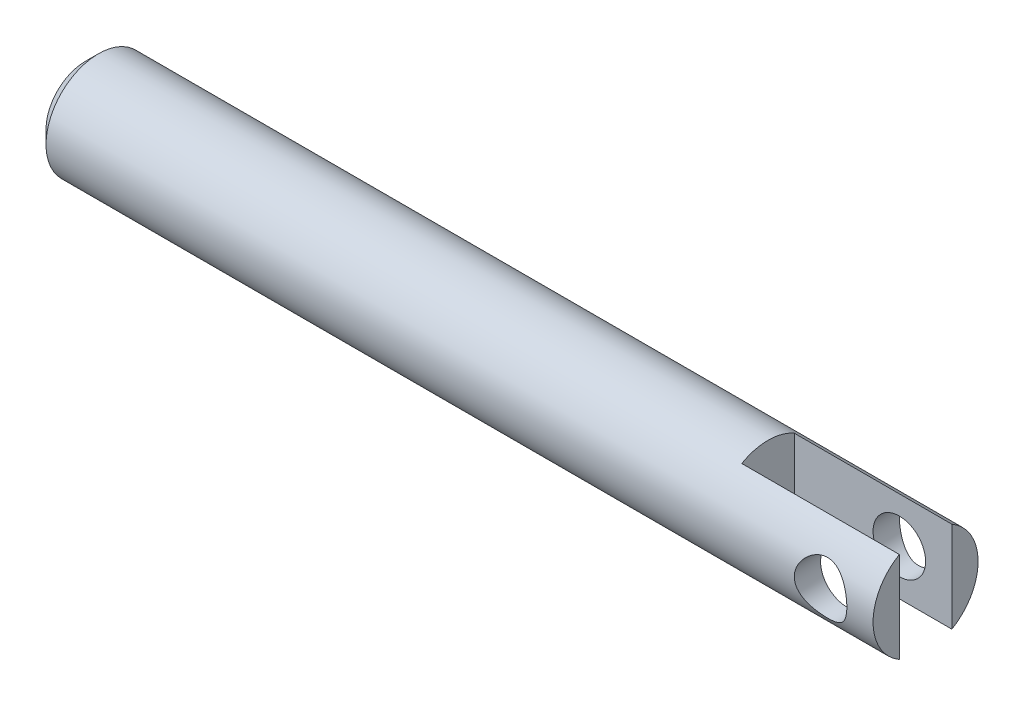
ISO-10303-21;
HEADER;
FILE_DESCRIPTION(('STEP AP214'),'2;1');
FILE_NAME('part.step','',(''),(''),'','','');
FILE_SCHEMA(('AUTOMOTIVE_DESIGN { 1 0 10303 214 1 1 1 1 }'));
ENDSEC;
DATA;
#1=APPLICATION_CONTEXT('core data for automotive mechanical design processes');
#2=APPLICATION_PROTOCOL_DEFINITION('international standard','automotive_design',2000,#1);
#3=PRODUCT_CONTEXT('',#1,'mechanical');
#4=PRODUCT('Part','Part','',(#3));
#5=PRODUCT_RELATED_PRODUCT_CATEGORY('part','',(#4));
#6=PRODUCT_DEFINITION_FORMATION('','',#4);
#7=PRODUCT_DEFINITION_CONTEXT('part definition',#1,'design');
#8=PRODUCT_DEFINITION('design','',#6,#7);
#9=PRODUCT_DEFINITION_SHAPE('','',#8);
#10=(LENGTH_UNIT() NAMED_UNIT(*) SI_UNIT(.MILLI.,.METRE.));
#11=(NAMED_UNIT(*) PLANE_ANGLE_UNIT() SI_UNIT($,.RADIAN.));
#12=(NAMED_UNIT(*) SI_UNIT($,.STERADIAN.) SOLID_ANGLE_UNIT());
#13=UNCERTAINTY_MEASURE_WITH_UNIT(LENGTH_MEASURE(1.E-05),#10,'distance_accuracy_value','');
#14=(GEOMETRIC_REPRESENTATION_CONTEXT(3) GLOBAL_UNCERTAINTY_ASSIGNED_CONTEXT((#13)) GLOBAL_UNIT_ASSIGNED_CONTEXT((#10,
#11,#12)) REPRESENTATION_CONTEXT('',''));
#15=CARTESIAN_POINT('',(0.,0.,0.));
#16=DIRECTION('',(0.,0.,1.));
#17=DIRECTION('',(1.,0.,0.));
#18=AXIS2_PLACEMENT_3D('',#15,#16,#17);
#19=CARTESIAN_POINT('',(50.8,6.35,0.));
#20=DIRECTION('',(-1.,0.,0.));
#21=DIRECTION('',(0.,0.,1.));
#22=AXIS2_PLACEMENT_3D('',#19,#20,#21);
#23=PLANE('',#22);
#24=CARTESIAN_POINT('',(50.8,0.,0.));
#25=DIRECTION('',(-1.,0.,0.));
#26=DIRECTION('',(0.,0.,1.));
#27=AXIS2_PLACEMENT_3D('',#24,#25,#26);
#28=CIRCLE('',#27,6.35);
#29=CARTESIAN_POINT('',(50.8,-5.49926131403119,3.175));
#30=VERTEX_POINT('',#29);
#31=CARTESIAN_POINT('',(50.8,5.49926131403119,3.175));
#32=VERTEX_POINT('',#31);
#33=EDGE_CURVE('E101',#30,#32,#28,.T.);
#34=ORIENTED_EDGE('',*,*,#33,.F.);
#35=DIRECTION('',(0.,1.,0.));
#36=VECTOR('',#35,1.);
#37=CARTESIAN_POINT('',(50.8,-127.,3.175));
#38=LINE('',#37,#36);
#39=EDGE_CURVE('E182',#30,#32,#38,.T.);
#40=ORIENTED_EDGE('',*,*,#39,.T.);
#41=EDGE_LOOP('',(#34,#40));
#42=FACE_BOUND('',#41,.T.);
#43=ADVANCED_FACE('F41',(#42),#23,.F.);
#44=CARTESIAN_POINT('',(44.45,0.,-127.));
#45=DIRECTION('',(0.,0.,1.));
#46=DIRECTION('',(1.,0.,0.));
#47=AXIS2_PLACEMENT_3D('',#44,#45,#46);
#48=CYLINDRICAL_SURFACE('',#47,3.175);
#49=CARTESIAN_POINT('',(44.45,0.,3.175));
#50=DIRECTION('',(0.,0.,1.));
#51=DIRECTION('',(1.,0.,0.));
#52=AXIS2_PLACEMENT_3D('',#49,#50,#51);
#53=CIRCLE('',#52,3.175);
#54=CARTESIAN_POINT('',(47.625,0.,3.175));
#55=VERTEX_POINT('',#54);
#56=EDGE_CURVE('E90',#55,#55,#53,.F.);
#57=ORIENTED_EDGE('',*,*,#56,.T.);
#58=EDGE_LOOP('',(#57));
#59=FACE_BOUND('',#58,.T.);
#60=CARTESIAN_POINT('',(47.625,0.,6.35));
#61=CARTESIAN_POINT('',(47.6249991122824,-0.0834969220595001,6.34999931166444));
#62=CARTESIAN_POINT('',(47.6217001255541,-0.167002655580043,6.34834758911701));
#63=CARTESIAN_POINT('',(47.6085541254501,-0.333378330258782,6.34179105821714));
#64=CARTESIAN_POINT('',(47.5987042634742,-0.416247978955772,6.33688483467113));
#65=CARTESIAN_POINT('',(47.559427934954,-0.66318203064701,6.31742426748325));
#66=CARTESIAN_POINT('',(47.5202749225986,-0.825450146761553,6.29812827299425));
#67=CARTESIAN_POINT('',(47.4180092887059,-1.13965128900426,6.2489182313574));
#68=CARTESIAN_POINT('',(47.3549897807566,-1.29162180811868,6.21904547786825));
#69=CARTESIAN_POINT('',(47.2072639263711,-1.58264035037879,6.15142812041637));
#70=CARTESIAN_POINT('',(47.1225592898491,-1.72168939123018,6.11368413715877));
#71=CARTESIAN_POINT('',(46.9280303702658,-1.99234108848171,6.03111096182982));
#72=CARTESIAN_POINT('',(46.8169964222061,-2.12298433900091,5.98599127270818));
#73=CARTESIAN_POINT('',(46.5756033164272,-2.36467069069853,5.89470535591056));
#74=CARTESIAN_POINT('',(46.4452295702336,-2.47569885601321,5.84853836069043));
#75=CARTESIAN_POINT('',(46.1565790522467,-2.68368848497886,5.75623634934464));
#76=CARTESIAN_POINT('',(45.9969224686984,-2.77889135161933,5.71038146176788));
#77=CARTESIAN_POINT('',(45.7454520128256,-2.90019349951534,5.64919759286363));
#78=CARTESIAN_POINT('',(45.6595999381713,-2.93705266116891,5.63006420805933));
#79=CARTESIAN_POINT('',(45.4844143862936,-3.00322508739606,5.59504604853268));
#80=CARTESIAN_POINT('',(45.3950830018195,-3.03254280972159,5.57915935583429));
#81=CARTESIAN_POINT('',(45.2189894480353,-3.08174263292982,5.55212611635049));
#82=CARTESIAN_POINT('',(45.1323892059714,-3.10208128111978,5.54075429137746));
#83=CARTESIAN_POINT('',(44.9574127210056,-3.13545600360765,5.52193654886444));
#84=CARTESIAN_POINT('',(44.8690374462283,-3.14849595237257,5.51448854851135));
#85=CARTESIAN_POINT('',(44.6912932611514,-3.1670771305344,5.50383875782919));
#86=CARTESIAN_POINT('',(44.6019249820126,-3.17262287599649,5.50063441026522));
#87=CARTESIAN_POINT('',(44.4230192158219,-3.17614778806993,5.49859788398609));
#88=CARTESIAN_POINT('',(44.3334817457287,-3.17412767659872,5.49976528812799));
#89=CARTESIAN_POINT('',(44.0872521242756,-3.1581193033026,5.50899190362733));
#90=CARTESIAN_POINT('',(43.9311582701866,-3.13621253452965,5.52160857357707));
#91=CARTESIAN_POINT('',(43.6253533586935,-3.07003746372167,5.55866493052824));
#92=CARTESIAN_POINT('',(43.4756443509772,-3.02576203854504,5.58310838358077));
#93=CARTESIAN_POINT('',(43.1824557034359,-2.91531509833647,5.64157885407237));
#94=CARTESIAN_POINT('',(43.0392023900634,-2.84865758129417,5.67581583876129));
#95=CARTESIAN_POINT('',(42.765233913826,-2.69570761526054,5.75003268807633));
#96=CARTESIAN_POINT('',(42.6345244203915,-2.60940634674629,5.79001512927804));
#97=CARTESIAN_POINT('',(42.3718957257497,-2.40685964249565,5.87734289018611));
#98=CARTESIAN_POINT('',(42.2419246151435,-2.28820488335253,5.92497898403936));
#99=CARTESIAN_POINT('',(42.0029148571362,-2.03058898448427,6.01813700574905));
#100=CARTESIAN_POINT('',(41.8938862136413,-1.89161819563546,6.06365791538158));
#101=CARTESIAN_POINT('',(41.6950980802803,-1.58913989972482,6.1500381059768));
#102=CARTESIAN_POINT('',(41.6064685144201,-1.42479265164789,6.19058274974572));
#103=CARTESIAN_POINT('',(41.4588419183647,-1.08098023585583,6.25976272299952));
#104=CARTESIAN_POINT('',(41.3998213588683,-0.901527205073898,6.28840750578946));
#105=CARTESIAN_POINT('',(41.317940596601,-0.548533610626836,6.32854759690358));
#106=CARTESIAN_POINT('',(41.2924903274127,-0.375734359385247,6.34126679122995));
#107=CARTESIAN_POINT('',(41.2703494777398,-0.0278752299448333,6.35231817716325));
#108=CARTESIAN_POINT('',(41.2736452728607,0.147183538060018,6.35065718436129));
#109=CARTESIAN_POINT('',(41.3074062359454,0.480164686080362,6.33384535408399));
#110=CARTESIAN_POINT('',(41.3357457914748,0.638363620564189,6.31975005060431));
#111=CARTESIAN_POINT('',(41.4154558782099,0.947441883053,6.28085393924121));
#112=CARTESIAN_POINT('',(41.4668289484773,1.09832040207141,6.25605195113515));
#113=CARTESIAN_POINT('',(41.5924951309378,1.39347133182512,6.19709998236334));
#114=CARTESIAN_POINT('',(41.6674015841112,1.53743151047821,6.16270299610718));
#115=CARTESIAN_POINT('',(41.8373164256859,1.8112148234104,6.08787118465665));
#116=CARTESIAN_POINT('',(41.9323333773854,1.94103189959927,6.0474337895468));
#117=CARTESIAN_POINT('',(42.1505393503738,2.19636241342679,5.95973602709939));
#118=CARTESIAN_POINT('',(42.2755786071116,2.3202013468198,5.91219559251098));
#119=CARTESIAN_POINT('',(42.5447623551498,2.54589381918873,5.81858093231368));
#120=CARTESIAN_POINT('',(42.6889199523809,2.6477321493525,5.77250773963547));
#121=CARTESIAN_POINT('',(43.0010686019584,2.83117262876715,5.68487535288742));
#122=CARTESIAN_POINT('',(43.1698757695104,2.91155594998013,5.64364281441821));
#123=CARTESIAN_POINT('',(43.5213444648897,3.04191297152938,5.5744767953732));
#124=CARTESIAN_POINT('',(43.7039877978474,3.09192585492219,5.54652618900869));
#125=CARTESIAN_POINT('',(44.0591899564702,3.15551086037918,5.51057765714603));
#126=CARTESIAN_POINT('',(44.2310337504072,3.17212027309711,5.50092192343245));
#127=CARTESIAN_POINT('',(44.5752444424952,3.17718805563876,5.49800001145358));
#128=CARTESIAN_POINT('',(44.7476110815426,3.16565862768385,5.5047267290444));
#129=CARTESIAN_POINT('',(45.0706601030739,3.11761548073658,5.53205211477784));
#130=CARTESIAN_POINT('',(45.2218439417312,3.08358651207686,5.55126823076269));
#131=CARTESIAN_POINT('',(45.5161908301672,2.99458164828807,5.59977978302582));
#132=CARTESIAN_POINT('',(45.6593512828503,2.93959901505999,5.62907846127335));
#133=CARTESIAN_POINT('',(45.9442336994286,2.8061154442137,5.69685576337174));
#134=CARTESIAN_POINT('',(46.0852128093657,2.72628260503929,5.73581889480533));
#135=CARTESIAN_POINT('',(46.3526974317231,2.54682759156583,5.81772207082382));
#136=CARTESIAN_POINT('',(46.4791953599427,2.44719512169931,5.8606641782013));
#137=CARTESIAN_POINT('',(46.7300975241771,2.21680287661218,5.95192753761204));
#138=CARTESIAN_POINT('',(46.8523797564128,2.08373188558712,6.00026839877346));
#139=CARTESIAN_POINT('',(47.0733978732331,1.79751265125243,6.0921234557675));
#140=CARTESIAN_POINT('',(47.1721210659827,1.64435365457428,6.13563504323043));
#141=CARTESIAN_POINT('',(47.3002802661971,1.40178715704487,6.19391073190243));
#142=CARTESIAN_POINT('',(47.3398005836814,1.31842200030918,6.21223173271383));
#143=CARTESIAN_POINT('',(47.4115994748237,1.1480770102167,6.24595363475604));
#144=CARTESIAN_POINT('',(47.4438816065344,1.06109897786306,6.26135597012704));
#145=CARTESIAN_POINT('',(47.500759345915,0.884361322813108,6.28875097111981));
#146=CARTESIAN_POINT('',(47.5253717181381,0.794608244970572,6.30075106809478));
#147=CARTESIAN_POINT('',(47.5666673895299,0.612925661591583,6.32100983571903));
#148=CARTESIAN_POINT('',(47.5833555321936,0.520997521680291,6.3292707916836));
#149=CARTESIAN_POINT('',(47.6056162848624,0.357531347524375,6.34032503263334));
#150=CARTESIAN_POINT('',(47.6128788212496,0.286274046488596,6.34394670812889));
#151=CARTESIAN_POINT('',(47.6225711265376,0.143346668941346,6.34878452045567));
#152=CARTESIAN_POINT('',(47.6250007620468,0.0716765810914255,6.35000059089052));
#153=CARTESIAN_POINT('',(47.625,0.,6.35));
#154=B_SPLINE_CURVE_WITH_KNOTS('',3,(#60,#61,#62,#63,#64,#65,#66,#67,#68,#69,#70,#71,#72,#73,
#74,#75,#76,#77,#78,#79,#80,#81,#82,#83,#84,#85,#86,#87,#88,#89,#90,#91,#92,#93,#94,#95,#96,#97,
#98,#99,#100,#101,#102,#103,#104,#105,#106,#107,#108,#109,#110,#111,#112,#113,#114,#115,#116,
#117,#118,#119,#120,#121,#122,#123,#124,#125,#126,#127,#128,#129,#130,#131,#132,#133,#134,#135,
#136,#137,#138,#139,#140,#141,#142,#143,#144,#145,#146,#147,#148,#149,#150,#151,#152,#153),
.UNSPECIFIED.,.T.,.F.,(4,2,2,2,2,2,2,2,2,2,2,2,2,2,2,2,2,2,2,2,2,2,2,2,2,2,2,2,2,2,2,2,2,2,2,2,
2,2,2,2,2,2,2,2,2,2,4),(0.,0.25041561210268,0.500940186864015,1.00234854488129,1.50182051324263,
2.00125310940106,2.53090025348451,3.06094897410615,3.63210298373097,3.91787290005988,
4.20347350732849,4.47213270490101,4.74064915090146,5.00900371453886,5.27733267302576,
5.74927594687738,6.22136960256845,6.70445970327764,7.18776712794021,7.7323564652788,
8.27720530143645,8.84735553323665,9.41705196489304,9.93956405039338,10.4618285011675,
10.9436138594975,11.4254523397102,11.9210677568139,12.4168946391879,12.9614122158798,
13.5063050164601,14.0775857365549,14.6481278321882,15.1639000911419,15.6794487286237,
16.1458838633213,16.6124691169503,17.1104020806943,17.6085946442304,18.1673210354482,
18.7263477502426,19.0082017078365,19.2899168101042,19.5710117490933,19.8519346536844,
20.0668939492148,20.2818591776892),.UNSPECIFIED.);
#155=CARTESIAN_POINT('',(47.625,0.,6.35));
#156=VERTEX_POINT('',#155);
#157=EDGE_CURVE('E106',#156,#156,#154,.T.);
#158=ORIENTED_EDGE('',*,*,#157,.F.);
#159=EDGE_LOOP('',(#158));
#160=FACE_BOUND('',#159,.T.);
#161=ADVANCED_FACE('F128',(#59,#160),#48,.F.);
#162=CARTESIAN_POINT('',(-50.8,6.35,0.));
#163=DIRECTION('',(1.,0.,0.));
#164=DIRECTION('',(0.,0.,-1.));
#165=AXIS2_PLACEMENT_3D('',#162,#163,#164);
#166=PLANE('',#165);
#167=CARTESIAN_POINT('',(-50.8,0.,0.));
#168=DIRECTION('',(1.,0.,0.));
#169=DIRECTION('',(0.,0.,-1.));
#170=AXIS2_PLACEMENT_3D('',#167,#168,#169);
#171=CIRCLE('',#170,4.76249999999999);
#172=CARTESIAN_POINT('',(-50.8,0.,-4.76249999999999));
#173=VERTEX_POINT('',#172);
#174=EDGE_CURVE('E47',#173,#173,#171,.F.);
#175=ORIENTED_EDGE('',*,*,#174,.T.);
#176=EDGE_LOOP('',(#175));
#177=FACE_BOUND('',#176,.T.);
#178=CARTESIAN_POINT('',(-50.8,0.,0.));
#179=DIRECTION('',(-1.,0.,0.));
#180=DIRECTION('',(0.,0.,1.));
#181=AXIS2_PLACEMENT_3D('',#178,#179,#180);
#182=CIRCLE('',#181,3.96875);
#183=CARTESIAN_POINT('',(-50.8,0.,3.96875));
#184=VERTEX_POINT('',#183);
#185=EDGE_CURVE('E176',#184,#184,#182,.T.);
#186=ORIENTED_EDGE('',*,*,#185,.F.);
#187=EDGE_LOOP('',(#186));
#188=FACE_BOUND('',#187,.T.);
#189=ADVANCED_FACE('F157',(#177,#188),#166,.F.);
#190=CARTESIAN_POINT('',(50.8,5.49926131403119,-3.175));
#191=VERTEX_POINT('',#190);
#192=CARTESIAN_POINT('',(50.8,-5.49926131403119,-3.175));
#193=VERTEX_POINT('',#192);
#194=EDGE_CURVE('E92',#191,#193,#28,.T.);
#195=ORIENTED_EDGE('',*,*,#194,.F.);
#196=DIRECTION('',(0.,1.,0.));
#197=VECTOR('',#196,1.);
#198=CARTESIAN_POINT('',(50.8,-127.,-3.175));
#199=LINE('',#198,#197);
#200=EDGE_CURVE('E57',#193,#191,#199,.T.);
#201=ORIENTED_EDGE('',*,*,#200,.F.);
#202=EDGE_LOOP('',(#195,#201));
#203=FACE_BOUND('',#202,.T.);
#204=ADVANCED_FACE('F94',(#203),#23,.F.);
#205=CARTESIAN_POINT('',(-58.2524572001112,0.,0.));
#206=DIRECTION('',(-1.,0.,0.));
#207=DIRECTION('',(0.,0.,1.));
#208=AXIS2_PLACEMENT_3D('',#205,#206,#207);
#209=CYLINDRICAL_SURFACE('',#208,6.35);
#210=CARTESIAN_POINT('',(-49.2125,0.,0.));
#211=DIRECTION('',(1.,0.,0.));
#212=DIRECTION('',(0.,0.,-1.));
#213=AXIS2_PLACEMENT_3D('',#210,#211,#212);
#214=CIRCLE('',#213,6.35);
#215=CARTESIAN_POINT('',(-49.2125,0.,-6.35));
#216=VERTEX_POINT('',#215);
#217=EDGE_CURVE('E11',#216,#216,#214,.T.);
#218=ORIENTED_EDGE('',*,*,#217,.T.);
#219=EDGE_LOOP('',(#218));
#220=FACE_BOUND('',#219,.T.);
#221=ORIENTED_EDGE('',*,*,#157,.T.);
#222=EDGE_LOOP('',(#221));
#223=FACE_BOUND('',#222,.T.);
#224=CARTESIAN_POINT('',(47.625,0.,-6.35));
#225=CARTESIAN_POINT('',(47.6249991122824,0.0834969220594997,-6.34999931166444));
#226=CARTESIAN_POINT('',(47.6217001255541,0.167002655580042,-6.34834758911701));
#227=CARTESIAN_POINT('',(47.6085541254501,0.333378330258781,-6.34179105821715));
#228=CARTESIAN_POINT('',(47.5987042634742,0.416247978955771,-6.33688483467113));
#229=CARTESIAN_POINT('',(47.559427934954,0.663182030647009,-6.31742426748325));
#230=CARTESIAN_POINT('',(47.5202749225986,0.825450146761553,-6.29812827299425));
#231=CARTESIAN_POINT('',(47.4180092887059,1.13965128900426,-6.2489182313574));
#232=CARTESIAN_POINT('',(47.3549897807566,1.29162180811868,-6.21904547786825));
#233=CARTESIAN_POINT('',(47.2072639263711,1.58264035037879,-6.15142812041637));
#234=CARTESIAN_POINT('',(47.1225592898491,1.72168939123018,-6.11368413715877));
#235=CARTESIAN_POINT('',(46.9280303702658,1.99234108848171,-6.03111096182982));
#236=CARTESIAN_POINT('',(46.8169964222061,2.12298433900091,-5.98599127270818));
#237=CARTESIAN_POINT('',(46.5756033164272,2.36467069069853,-5.89470535591056));
#238=CARTESIAN_POINT('',(46.4452295702336,2.47569885601321,-5.84853836069043));
#239=CARTESIAN_POINT('',(46.1565790522467,2.68368848497886,-5.75623634934464));
#240=CARTESIAN_POINT('',(45.9969224686984,2.77889135161933,-5.71038146176788));
#241=CARTESIAN_POINT('',(45.7454520128256,2.90019349951534,-5.64919759286363));
#242=CARTESIAN_POINT('',(45.6595999381713,2.93705266116891,-5.63006420805933));
#243=CARTESIAN_POINT('',(45.4844143862936,3.00322508739606,-5.59504604853268));
#244=CARTESIAN_POINT('',(45.3950830018195,3.03254280972159,-5.57915935583429));
#245=CARTESIAN_POINT('',(45.2189894480353,3.08174263292982,-5.55212611635049));
#246=CARTESIAN_POINT('',(45.1323892059714,3.10208128111978,-5.54075429137746));
#247=CARTESIAN_POINT('',(44.9574127210056,3.13545600360765,-5.52193654886444));
#248=CARTESIAN_POINT('',(44.8690374462283,3.14849595237257,-5.51448854851135));
#249=CARTESIAN_POINT('',(44.6912932611514,3.1670771305344,-5.50383875782919));
#250=CARTESIAN_POINT('',(44.6019249820126,3.17262287599649,-5.50063441026522));
#251=CARTESIAN_POINT('',(44.4230192158219,3.17614778806993,-5.49859788398609));
#252=CARTESIAN_POINT('',(44.3334817457287,3.17412767659872,-5.49976528812799));
#253=CARTESIAN_POINT('',(44.0872521242756,3.1581193033026,-5.50899190362733));
#254=CARTESIAN_POINT('',(43.9311582701866,3.13621253452965,-5.52160857357707));
#255=CARTESIAN_POINT('',(43.6253533586935,3.07003746372167,-5.55866493052824));
#256=CARTESIAN_POINT('',(43.4756443509772,3.02576203854504,-5.58310838358077));
#257=CARTESIAN_POINT('',(43.1824557034359,2.91531509833647,-5.64157885407237));
#258=CARTESIAN_POINT('',(43.0392023900634,2.84865758129417,-5.67581583876129));
#259=CARTESIAN_POINT('',(42.765233913826,2.69570761526054,-5.75003268807633));
#260=CARTESIAN_POINT('',(42.6345244203915,2.60940634674629,-5.79001512927804));
#261=CARTESIAN_POINT('',(42.3718957257497,2.40685964249565,-5.87734289018611));
#262=CARTESIAN_POINT('',(42.2419246151435,2.28820488335253,-5.92497898403936));
#263=CARTESIAN_POINT('',(42.0029148571362,2.03058898448427,-6.01813700574905));
#264=CARTESIAN_POINT('',(41.8938862136413,1.89161819563546,-6.06365791538158));
#265=CARTESIAN_POINT('',(41.6950980802803,1.58913989972482,-6.1500381059768));
#266=CARTESIAN_POINT('',(41.6064685144201,1.42479265164789,-6.19058274974572));
#267=CARTESIAN_POINT('',(41.4588419183647,1.08098023585583,-6.25976272299952));
#268=CARTESIAN_POINT('',(41.3998213588683,0.901527205073898,-6.28840750578946));
#269=CARTESIAN_POINT('',(41.317940596601,0.548533610626835,-6.32854759690358));
#270=CARTESIAN_POINT('',(41.2924903274127,0.375734359385245,-6.34126679122995));
#271=CARTESIAN_POINT('',(41.2703494777398,0.0278752299448316,-6.35231817716325));
#272=CARTESIAN_POINT('',(41.2736452728607,-0.147183538060019,-6.35065718436129));
#273=CARTESIAN_POINT('',(41.3074062359454,-0.480164686080362,-6.33384535408399));
#274=CARTESIAN_POINT('',(41.3357457914748,-0.63836362056419,-6.31975005060431));
#275=CARTESIAN_POINT('',(41.4154558782099,-0.947441883053001,-6.28085393924121));
#276=CARTESIAN_POINT('',(41.4668289484773,-1.09832040207141,-6.25605195113515));
#277=CARTESIAN_POINT('',(41.5924951309378,-1.39347133182512,-6.19709998236334));
#278=CARTESIAN_POINT('',(41.6674015841112,-1.53743151047822,-6.16270299610718));
#279=CARTESIAN_POINT('',(41.8373164256859,-1.8112148234104,-6.08787118465664));
#280=CARTESIAN_POINT('',(41.9323333773854,-1.94103189959927,-6.0474337895468));
#281=CARTESIAN_POINT('',(42.1505393503738,-2.19636241342679,-5.95973602709939));
#282=CARTESIAN_POINT('',(42.2755786071116,-2.3202013468198,-5.91219559251098));
#283=CARTESIAN_POINT('',(42.5447623551498,-2.54589381918874,-5.81858093231368));
#284=CARTESIAN_POINT('',(42.6889199523809,-2.64773214935251,-5.77250773963547));
#285=CARTESIAN_POINT('',(43.0010686019584,-2.83117262876716,-5.68487535288742));
#286=CARTESIAN_POINT('',(43.1698757695104,-2.91155594998014,-5.64364281441821));
#287=CARTESIAN_POINT('',(43.5213444648897,-3.04191297152938,-5.5744767953732));
#288=CARTESIAN_POINT('',(43.7039877978474,-3.09192585492219,-5.54652618900869));
#289=CARTESIAN_POINT('',(44.0591899564702,-3.15551086037918,-5.51057765714603));
#290=CARTESIAN_POINT('',(44.2310337504072,-3.17212027309711,-5.50092192343245));
#291=CARTESIAN_POINT('',(44.5752444424952,-3.17718805563876,-5.49800001145358));
#292=CARTESIAN_POINT('',(44.7476110815427,-3.16565862768385,-5.50472672904441));
#293=CARTESIAN_POINT('',(45.0706601030739,-3.11761548073657,-5.53205211477784));
#294=CARTESIAN_POINT('',(45.2218439417312,-3.08358651207686,-5.55126823076269));
#295=CARTESIAN_POINT('',(45.5161908301672,-2.99458164828807,-5.59977978302582));
#296=CARTESIAN_POINT('',(45.6593512828503,-2.93959901505999,-5.62907846127335));
#297=CARTESIAN_POINT('',(45.9442336994286,-2.8061154442137,-5.69685576337174));
#298=CARTESIAN_POINT('',(46.0852128093657,-2.72628260503929,-5.73581889480533));
#299=CARTESIAN_POINT('',(46.3526974317231,-2.54682759156583,-5.81772207082382));
#300=CARTESIAN_POINT('',(46.4791953599427,-2.44719512169931,-5.8606641782013));
#301=CARTESIAN_POINT('',(46.7300975241771,-2.21680287661218,-5.95192753761204));
#302=CARTESIAN_POINT('',(46.8523797564128,-2.08373188558712,-6.00026839877347));
#303=CARTESIAN_POINT('',(47.0733978732331,-1.79751265125243,-6.0921234557675));
#304=CARTESIAN_POINT('',(47.1721210659827,-1.64435365457428,-6.13563504323043));
#305=CARTESIAN_POINT('',(47.3002802661971,-1.40178715704487,-6.19391073190243));
#306=CARTESIAN_POINT('',(47.3398005836814,-1.31842200030918,-6.21223173271383));
#307=CARTESIAN_POINT('',(47.4115994748237,-1.1480770102167,-6.24595363475604));
#308=CARTESIAN_POINT('',(47.4438816065344,-1.06109897786306,-6.26135597012704));
#309=CARTESIAN_POINT('',(47.500759345915,-0.884361322813107,-6.28875097111981));
#310=CARTESIAN_POINT('',(47.5253717181381,-0.79460824497057,-6.30075106809478));
#311=CARTESIAN_POINT('',(47.5666673895299,-0.61292566159158,-6.32100983571903));
#312=CARTESIAN_POINT('',(47.5833555321936,-0.520997521680289,-6.3292707916836));
#313=CARTESIAN_POINT('',(47.6056162848624,-0.357531347524375,-6.34032503263334));
#314=CARTESIAN_POINT('',(47.6128788212496,-0.286274046488597,-6.34394670812889));
#315=CARTESIAN_POINT('',(47.6225711265376,-0.143346668941348,-6.34878452045567));
#316=CARTESIAN_POINT('',(47.6250007620468,-0.0716765810914264,-6.35000059089052));
#317=CARTESIAN_POINT('',(47.625,0.,-6.35));
#318=B_SPLINE_CURVE_WITH_KNOTS('',3,(#224,#225,#226,#227,#228,#229,#230,#231,#232,#233,#234,
#235,#236,#237,#238,#239,#240,#241,#242,#243,#244,#245,#246,#247,#248,#249,#250,#251,#252,#253,
#254,#255,#256,#257,#258,#259,#260,#261,#262,#263,#264,#265,#266,#267,#268,#269,#270,#271,#272,
#273,#274,#275,#276,#277,#278,#279,#280,#281,#282,#283,#284,#285,#286,#287,#288,#289,#290,#291,
#292,#293,#294,#295,#296,#297,#298,#299,#300,#301,#302,#303,#304,#305,#306,#307,#308,#309,#310,
#311,#312,#313,#314,#315,#316,#317),.UNSPECIFIED.,.T.,.F.,(4,2,2,2,2,2,2,2,2,2,2,2,2,2,2,2,2,2,
2,2,2,2,2,2,2,2,2,2,2,2,2,2,2,2,2,2,2,2,2,2,2,2,2,2,2,2,4),(0.,0.25041561210268,
0.500940186864013,1.00234854488129,1.50182051324263,2.00125310940106,2.53090025348452,
3.06094897410615,3.63210298373097,3.91787290005988,4.20347350732849,4.47213270490101,
4.74064915090146,5.00900371453886,5.27733267302576,5.74927594687738,6.22136960256845,
6.70445970327764,7.18776712794021,7.7323564652788,8.27720530143645,8.84735553323665,
9.41705196489304,9.93956405039339,10.4618285011675,10.9436138594975,11.4254523397102,
11.9210677568139,12.4168946391879,12.9614122158798,13.5063050164601,14.0775857365549,
14.6481278321882,15.1639000911419,15.6794487286237,16.1458838633213,16.6124691169503,
17.1104020806943,17.6085946442304,18.1673210354482,18.7263477502426,19.0082017078365,
19.2899168101042,19.5710117490933,19.8519346536844,20.0668939492147,20.2818591776892),.UNSPECIFIED.);
#319=CARTESIAN_POINT('',(47.625,0.,-6.35));
#320=VERTEX_POINT('',#319);
#321=EDGE_CURVE('E109',#320,#320,#318,.T.);
#322=ORIENTED_EDGE('',*,*,#321,.T.);
#323=EDGE_LOOP('',(#322));
#324=FACE_BOUND('',#323,.T.);
#325=CARTESIAN_POINT('',(31.75,0.,0.));
#326=DIRECTION('',(-1.,0.,0.));
#327=DIRECTION('',(0.,0.,1.));
#328=AXIS2_PLACEMENT_3D('',#325,#326,#327);
#329=CIRCLE('',#328,6.35);
#330=CARTESIAN_POINT('',(31.75,-5.49926131403119,-3.175));
#331=VERTEX_POINT('',#330);
#332=CARTESIAN_POINT('',(31.75,-5.49926131403118,3.175));
#333=VERTEX_POINT('',#332);
#334=EDGE_CURVE('E103',#331,#333,#329,.T.);
#335=ORIENTED_EDGE('',*,*,#334,.T.);
#336=DIRECTION('',(-1.,0.,0.));
#337=VECTOR('',#336,1.);
#338=CARTESIAN_POINT('',(-58.2524572001112,-5.49926131403118,3.175));
#339=LINE('',#338,#337);
#340=EDGE_CURVE('E190',#333,#30,#339,.F.);
#341=ORIENTED_EDGE('',*,*,#340,.T.);
#342=ORIENTED_EDGE('',*,*,#33,.T.);
#343=DIRECTION('',(-1.,0.,0.));
#344=VECTOR('',#343,1.);
#345=CARTESIAN_POINT('',(-58.2524572001112,5.49926131403118,3.175));
#346=LINE('',#345,#344);
#347=CARTESIAN_POINT('',(31.75,5.49926131403118,3.175));
#348=VERTEX_POINT('',#347);
#349=EDGE_CURVE('E64',#32,#348,#346,.T.);
#350=ORIENTED_EDGE('',*,*,#349,.T.);
#351=CARTESIAN_POINT('',(31.75,5.49926131403119,-3.175));
#352=VERTEX_POINT('',#351);
#353=EDGE_CURVE('E99',#348,#352,#329,.T.);
#354=ORIENTED_EDGE('',*,*,#353,.T.);
#355=DIRECTION('',(-1.,0.,0.));
#356=VECTOR('',#355,1.);
#357=CARTESIAN_POINT('',(-58.2524572001112,5.49926131403119,-3.175));
#358=LINE('',#357,#356);
#359=EDGE_CURVE('E89',#352,#191,#358,.F.);
#360=ORIENTED_EDGE('',*,*,#359,.T.);
#361=ORIENTED_EDGE('',*,*,#194,.T.);
#362=DIRECTION('',(-1.,0.,0.));
#363=VECTOR('',#362,1.);
#364=CARTESIAN_POINT('',(-58.2524572001112,-5.49926131403119,-3.175));
#365=LINE('',#364,#363);
#366=EDGE_CURVE('E85',#193,#331,#365,.T.);
#367=ORIENTED_EDGE('',*,*,#366,.T.);
#368=EDGE_LOOP('',(#335,#341,#342,#350,#354,#360,#361,#367));
#369=FACE_BOUND('',#368,.T.);
#370=ADVANCED_FACE('F98',(#220,#223,#324,#369),#209,.T.);
#371=CARTESIAN_POINT('',(44.45,0.,-3.175));
#372=DIRECTION('',(0.,0.,-1.));
#373=DIRECTION('',(-1.,0.,0.));
#374=AXIS2_PLACEMENT_3D('',#371,#372,#373);
#375=CIRCLE('',#374,3.175);
#376=CARTESIAN_POINT('',(41.275,0.,-3.175));
#377=VERTEX_POINT('',#376);
#378=EDGE_CURVE('E181',#377,#377,#375,.F.);
#379=ORIENTED_EDGE('',*,*,#378,.T.);
#380=EDGE_LOOP('',(#379));
#381=FACE_BOUND('',#380,.T.);
#382=ORIENTED_EDGE('',*,*,#321,.F.);
#383=EDGE_LOOP('',(#382));
#384=FACE_BOUND('',#383,.T.);
#385=ADVANCED_FACE('F123',(#381,#384),#48,.F.);
#386=CARTESIAN_POINT('',(31.75,-127.,3.175));
#387=DIRECTION('',(-1.,0.,0.));
#388=DIRECTION('',(0.,0.,1.));
#389=AXIS2_PLACEMENT_3D('',#386,#387,#388);
#390=PLANE('',#389);
#391=DIRECTION('',(0.,1.,0.));
#392=VECTOR('',#391,1.);
#393=CARTESIAN_POINT('',(31.75,-127.,3.175));
#394=LINE('',#393,#392);
#395=EDGE_CURVE('E184',#333,#348,#394,.T.);
#396=ORIENTED_EDGE('',*,*,#395,.F.);
#397=ORIENTED_EDGE('',*,*,#334,.F.);
#398=DIRECTION('',(0.,1.,0.));
#399=VECTOR('',#398,1.);
#400=CARTESIAN_POINT('',(31.75,-127.,-3.175));
#401=LINE('',#400,#399);
#402=EDGE_CURVE('E84',#331,#352,#401,.T.);
#403=ORIENTED_EDGE('',*,*,#402,.T.);
#404=ORIENTED_EDGE('',*,*,#353,.F.);
#405=EDGE_LOOP('',(#396,#397,#403,#404));
#406=FACE_BOUND('',#405,.T.);
#407=ADVANCED_FACE('F126',(#406),#390,.F.);
#408=CARTESIAN_POINT('',(31.75,-127.,3.175));
#409=DIRECTION('',(0.,0.,1.));
#410=DIRECTION('',(1.,0.,0.));
#411=AXIS2_PLACEMENT_3D('',#408,#409,#410);
#412=PLANE('',#411);
#413=ORIENTED_EDGE('',*,*,#56,.F.);
#414=EDGE_LOOP('',(#413));
#415=FACE_BOUND('',#414,.T.);
#416=ORIENTED_EDGE('',*,*,#39,.F.);
#417=ORIENTED_EDGE('',*,*,#340,.F.);
#418=ORIENTED_EDGE('',*,*,#395,.T.);
#419=ORIENTED_EDGE('',*,*,#349,.F.);
#420=EDGE_LOOP('',(#416,#417,#418,#419));
#421=FACE_BOUND('',#420,.T.);
#422=ADVANCED_FACE('F132',(#415,#421),#412,.F.);
#423=CARTESIAN_POINT('',(31.75,-127.,-3.175));
#424=DIRECTION('',(0.,0.,-1.));
#425=DIRECTION('',(-1.,0.,0.));
#426=AXIS2_PLACEMENT_3D('',#423,#424,#425);
#427=PLANE('',#426);
#428=ORIENTED_EDGE('',*,*,#378,.F.);
#429=EDGE_LOOP('',(#428));
#430=FACE_BOUND('',#429,.T.);
#431=ORIENTED_EDGE('',*,*,#200,.T.);
#432=ORIENTED_EDGE('',*,*,#359,.F.);
#433=ORIENTED_EDGE('',*,*,#402,.F.);
#434=ORIENTED_EDGE('',*,*,#366,.F.);
#435=EDGE_LOOP('',(#431,#432,#433,#434));
#436=FACE_BOUND('',#435,.T.);
#437=ADVANCED_FACE('F82',(#430,#436),#427,.F.);
#438=CARTESIAN_POINT('',(-6.35,0.,0.));
#439=DIRECTION('',(-1.,0.,0.));
#440=DIRECTION('',(0.,0.,1.));
#441=AXIS2_PLACEMENT_3D('',#438,#439,#440);
#442=CYLINDRICAL_SURFACE('',#441,3.96875);
#443=CARTESIAN_POINT('',(-6.35,0.,0.));
#444=DIRECTION('',(-1.,0.,0.));
#445=DIRECTION('',(0.,0.,1.));
#446=AXIS2_PLACEMENT_3D('',#443,#444,#445);
#447=CIRCLE('',#446,3.96875);
#448=CARTESIAN_POINT('',(-6.35,0.,3.96875));
#449=VERTEX_POINT('',#448);
#450=EDGE_CURVE('E96',#449,#449,#447,.T.);
#451=ORIENTED_EDGE('',*,*,#450,.F.);
#452=EDGE_LOOP('',(#451));
#453=FACE_BOUND('',#452,.T.);
#454=ORIENTED_EDGE('',*,*,#185,.T.);
#455=EDGE_LOOP('',(#454));
#456=FACE_BOUND('',#455,.T.);
#457=ADVANCED_FACE('F134',(#453,#456),#442,.F.);
#458=CARTESIAN_POINT('',(-6.35,0.,0.));
#459=DIRECTION('',(-1.,0.,0.));
#460=DIRECTION('',(0.,0.,1.));
#461=AXIS2_PLACEMENT_3D('',#458,#459,#460);
#462=PLANE('',#461);
#463=ORIENTED_EDGE('',*,*,#450,.T.);
#464=EDGE_LOOP('',(#463));
#465=FACE_BOUND('',#464,.T.);
#466=ADVANCED_FACE('F144',(#465),#462,.T.);
#467=CARTESIAN_POINT('',(-50.8,0.,0.));
#468=DIRECTION('',(1.,0.,0.));
#469=DIRECTION('',(0.,0.,-1.));
#470=AXIS2_PLACEMENT_3D('',#467,#468,#469);
#471=CONICAL_SURFACE('',#470,4.76249999999999,0.785398163397445);
#472=ORIENTED_EDGE('',*,*,#217,.F.);
#473=EDGE_LOOP('',(#472));
#474=FACE_BOUND('',#473,.T.);
#475=ORIENTED_EDGE('',*,*,#174,.F.);
#476=EDGE_LOOP('',(#475));
#477=FACE_BOUND('',#476,.T.);
#478=ADVANCED_FACE('F43',(#474,#477),#471,.T.);
#479=CLOSED_SHELL('',(#43,#161,#189,#204,#370,#385,#407,#422,#437,#457,#466,#478));
#480=MANIFOLD_SOLID_BREP('B2',#479);
#481=ADVANCED_BREP_SHAPE_REPRESENTATION('',(#18,#480),#14);
#482=SHAPE_DEFINITION_REPRESENTATION(#9,#481);
ENDSEC;
END-ISO-10303-21;
